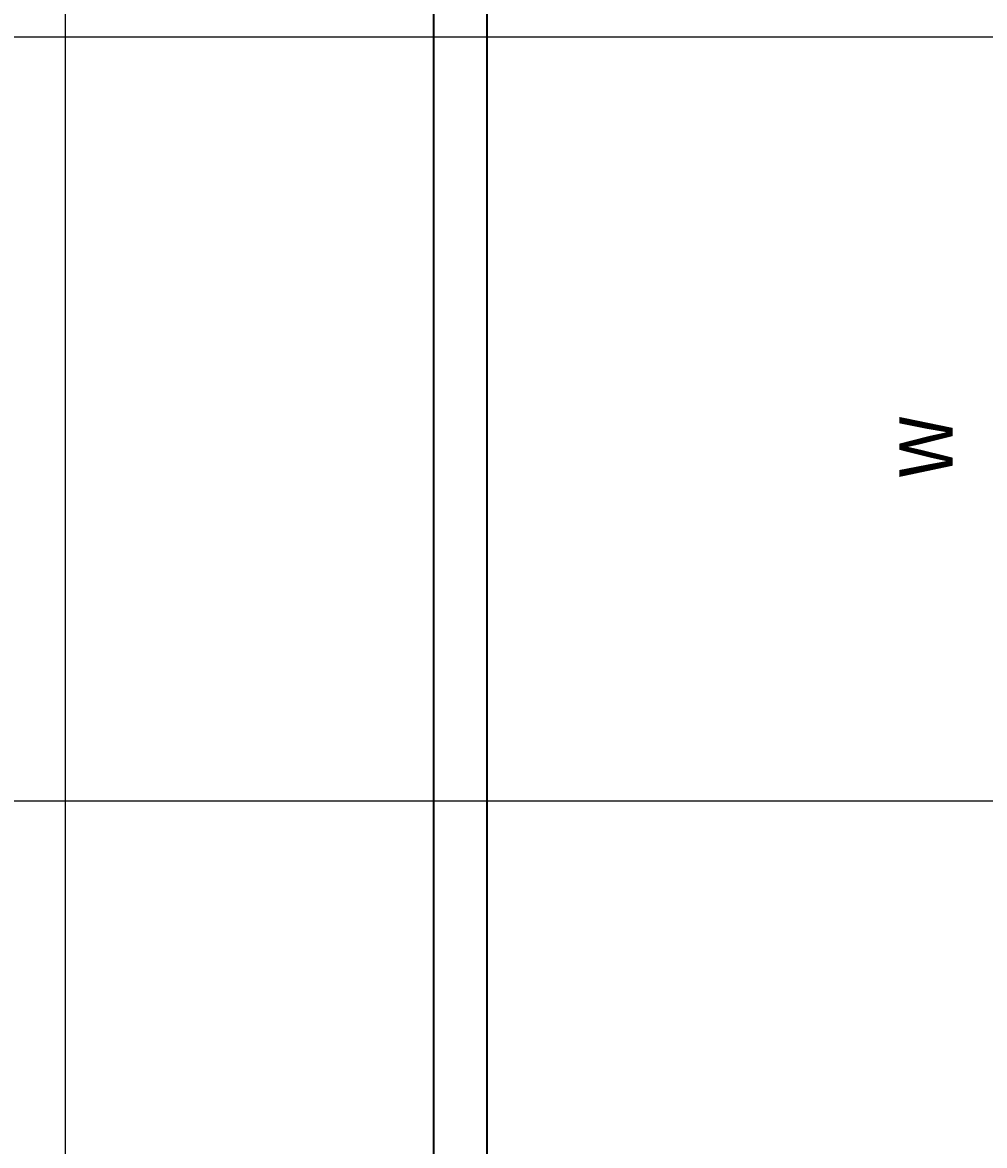
# Model space of a CAD drawing. Units: inches. Extents: x -364 to 705, y -52 to 1250.
# Tile 21 of 34: x -134 to 29, y 648 to 838. Entities that reach past the tile are written whole.
import ezdxf

# ---------------------------------------------------------------- set-up
doc = ezdxf.new("R2010")
doc.units = ezdxf.units.IN
doc.header["$MEASUREMENT"] = 0
for name, color, linetype, lineweight in [('A-ANNO-DIMS', 4, 'Continuous', 18), ('A-ANNO-IDEN', 1, 'Continuous', 18), ('C-WALL', 41, 'Continuous', 35)]:
    doc.layers.add(name, color=color, linetype=linetype, lineweight=lineweight)
doc.styles.get("Standard").update_dxf_attribs({"font": 'arial.ttf'})
doc.dimstyles.get("Standard").update_dxf_attribs({"dimtxt": 1, "dimasz": 1, "dimexe": 0.18, "dimexo": 0.0625, "dimgap": 0.09, "dimtad": 0, "dimtih": 1, "dimtoh": 1, "dimdec": 0, "dimzin": 0, "dimdsep": 46, "dimlunit": 3, "dimtxsty": 'Standard', "dimcen": 0.09, "dimadec": 0, "dimazin": 0, "dimtfac": 1, "dimtdec": 0, "dimtofl": 0, "dimtmove": 0, "dimatfit": 3, "dimfxl": 1, "dimtolj": 1, "dimtzin": 0, "dimarcsym": 0})

# ---------------------------------------------------------------- blocks, each defined once
blk = doc.blocks.new('*D19')
at = {"layer": 'A-ANNO-DIMS', "color": 0, "lineweight": -2, "transparency": 16777216}
for p, q in [((28.52, 986.11), (-248.33, 986.11)), ((-248.15, 985.11), (-248.15, 574.22)), ((-248.15, 149.87), (-248.15, 560.77)), ((28.52, 148.87), (-248.33, 148.87))]:
    blk.add_line(p, q, dxfattribs=at)
at = {"layer": 'A-ANNO-DIMS', "color": 0, "transparency": 16777216}
for points in [[(-248.32, 985.11), (-247.99, 985.11), (-248.15, 986.11)], [(-248.32, 149.87), (-247.99, 149.87), (-248.15, 148.87)]]:
    blk.add_solid(points, dxfattribs=at)
at = {"layer": 'Defpoints', "color": 0, "transparency": 16777216}
for p in [(28.58, 986.11), (-248.15, 148.87), (28.58, 148.87)]:
    blk.add_point(p, dxfattribs=at)
at = {"layer": 'A-ANNO-DIMS', "color": 0, "transparency": 16777216, "insert": (-248.15, 567.49), "char_height": 1, "attachment_point": 5}
blk.add_mtext('\\A1;{\\H13x;69\'-9"}', dxfattribs=at)
blk = doc.blocks.new('*D20')
at = {"layer": 'A-ANNO-DIMS', "color": 0, "lineweight": -2, "transparency": 16777216}
for p, q in [((28.52, 986.11), (-188.21, 986.11)), ((-188.03, 985.11), (-188.03, 917.23)), ((-188.03, 836.11), (-188.03, 904)), ((37.52, 835.11), (-188.21, 835.11))]:
    blk.add_line(p, q, dxfattribs=at)
at = {"layer": 'A-ANNO-DIMS', "color": 0, "transparency": 16777216}
for points in [[(-188.19, 985.11), (-187.86, 985.11), (-188.03, 986.11)], [(-188.19, 836.11), (-187.86, 836.11), (-188.03, 835.11)]]:
    blk.add_solid(points, dxfattribs=at)
at = {"layer": 'Defpoints', "color": 0, "transparency": 16777216}
for p in [(28.58, 986.11), (-188.03, 835.11), (37.58, 835.11)]:
    blk.add_point(p, dxfattribs=at)
at = {"layer": 'A-ANNO-DIMS', "color": 0, "transparency": 16777216, "insert": (-188.03, 910.61), "char_height": 1, "attachment_point": 5}
blk.add_mtext('\\A1;{\\H13x;12\'-7"}', dxfattribs=at)
blk = doc.blocks.new('*D21')
at = {"layer": 'A-ANNO-DIMS', "color": 0, "lineweight": -2, "transparency": 16777216}
for p, q in [((37.52, 835.11), (-188.94, 835.11)), ((-188.76, 834.11), (-188.76, 777.34)), ((-188.76, 707.11), (-188.76, 763.89)), ((37.52, 706.11), (-188.94, 706.11))]:
    blk.add_line(p, q, dxfattribs=at)
at = {"layer": 'A-ANNO-DIMS', "color": 0, "transparency": 16777216}
for points in [[(-188.93, 834.11), (-188.59, 834.11), (-188.76, 835.11)], [(-188.93, 707.11), (-188.59, 707.11), (-188.76, 706.11)]]:
    blk.add_solid(points, dxfattribs=at)
at = {"layer": 'Defpoints', "color": 0, "transparency": 16777216}
for p in [(37.58, 835.11), (-188.76, 706.11), (37.58, 706.11)]:
    blk.add_point(p, dxfattribs=at)
at = {"layer": 'A-ANNO-DIMS', "color": 0, "transparency": 16777216, "insert": (-188.76, 770.61), "char_height": 1, "attachment_point": 5}
blk.add_mtext('\\A1;{\\H13x;10\'-9"}', dxfattribs=at)
blk = doc.blocks.new('*D31')
at = {"layer": 'A-ANNO-DIMS', "color": 0, "lineweight": -2, "transparency": 16777216}
for p, q in [((37.52, 706.11), (-205.07, 706.11)), ((-204.89, 705.11), (-204.89, 648.34)), ((-204.89, 578.11), (-204.89, 634.89)), ((37.52, 577.11), (-205.07, 577.11))]:
    blk.add_line(p, q, dxfattribs=at)
at = {"layer": 'A-ANNO-DIMS', "color": 0, "transparency": 16777216}
for points in [[(-205.06, 705.11), (-204.73, 705.11), (-204.89, 706.11)], [(-205.06, 578.11), (-204.73, 578.11), (-204.89, 577.11)]]:
    blk.add_solid(points, dxfattribs=at)
at = {"layer": 'Defpoints', "color": 0, "transparency": 16777216}
for p in [(37.58, 706.11), (-204.89, 577.11), (37.58, 577.11)]:
    blk.add_point(p, dxfattribs=at)
at = {"layer": 'A-ANNO-DIMS', "color": 0, "transparency": 16777216, "insert": (-204.89, 641.61), "char_height": 1, "attachment_point": 5}
blk.add_mtext('\\A1;{\\H13x;10\'-9"}', dxfattribs=at)
blk = doc.blocks.new('*D76')
at = {"layer": 'A-ANNO-DIMS', "color": 0, "lineweight": -2, "transparency": 16777216}
for p, q in [((28.52, 986.11), (-126.85, 986.11)), ((-126.67, 985.11), (-126.67, 499.22)), ((-126.67, 12.11), (-126.67, 498.01)), ((28.52, 11.11), (-126.85, 11.11))]:
    blk.add_line(p, q, dxfattribs=at)
at = {"layer": 'A-ANNO-DIMS', "color": 0, "transparency": 16777216}
for points in [[(-126.84, 985.11), (-126.5, 985.11), (-126.67, 986.11)], [(-126.84, 12.11), (-126.5, 12.11), (-126.67, 11.11)]]:
    blk.add_solid(points, dxfattribs=at)
at = {"layer": 'Defpoints', "color": 0, "transparency": 16777216}
for p in [(-126.67, 986.11), (28.58, 986.11), (28.58, 11.11)]:
    blk.add_point(p, dxfattribs=at)
at = {"layer": 'A-ANNO-DIMS', "color": 0, "transparency": 16777216, "insert": (-126.67, 498.61), "char_height": 1, "attachment_point": 5}
blk.add_mtext('\\A1;81\'-3"', dxfattribs=at)

msp = doc.modelspace()

# ---------------------------------------------------------------- linework, layer by layer
at = {"layer": 'C-WALL'}
for p, q in [((-64.42, 11.11), (-64.42, 1079.11)), ((-55.42, 11.11), (-55.42, 1070.11))]:
    msp.add_line(p, q, dxfattribs=at)

# ---------------------------------------------------------------- texts
at = {"layer": 'A-ANNO-IDEN', "insert": (14.21, 760.54), "char_height": 9, "attachment_point": 1, "rotation": 90}
msp.add_mtext_dynamic_manual_height_columns('W', width=31.4151, gutter_width=1, heights=[0], dxfattribs=at)

# ---------------------------------------------------------------- dimensions: what is measured, and where the dimension line sits
at = {"layer": 'A-ANNO-DIMS'}
for base, p1, p2, picture, middle in [((-248.15, 148.87), (28.58, 986.11), (28.58, 148.87), '*D19', (-248.15, 567.49)), ((-188.76, 706.11), (37.58, 835.11), (37.58, 706.11), '*D21', (-188.76, 770.61)), ((-204.89, 577.11), (37.58, 706.11), (37.58, 577.11), '*D31', (-204.89, 641.61))]:
    dim = msp.add_linear_dim(base=base, p1=p1, p2=p2, angle=90, text='{\\H13x;<>}', dimstyle='Standard', override={"dimclrd": 0, "dimclre": 0, "dimclrt": 0}, dxfattribs=at)
    dim.commit()
    dim.dimension.update_dxf_attribs({"geometry": picture, "text_midpoint": middle})
dim = msp.add_linear_dim(base=(-188.03, 835.11), p1=(28.58, 986.11), p2=(37.58, 835.11), angle=90, text='{\\H13x;<>}', dimstyle='Standard', override={"dimclrd": 0, "dimclre": 0, "dimclrt": 0}, dxfattribs=at)
dim.commit()
dim.dimension.update_dxf_attribs({"geometry": '*D20', "text_midpoint": (-188.03, 910.61), "dimtype": 160})
dim = msp.add_linear_dim(base=(-126.67, 986.11), p1=(28.58, 11.11), p2=(28.58, 986.11), angle=90, dimstyle='Standard', override={"dimdec": 1, "dimlfac": 1, "dimrnd": 0, "dimzin": 1, "dimdsep": 46, "dimlunit": 4, "dimfrac": 2}, dxfattribs=at)
dim.commit()
dim.dimension.update_dxf_attribs({"geometry": '*D76', "text_midpoint": (-126.67, 498.61)})

doc.saveas('drawing.dxf')
